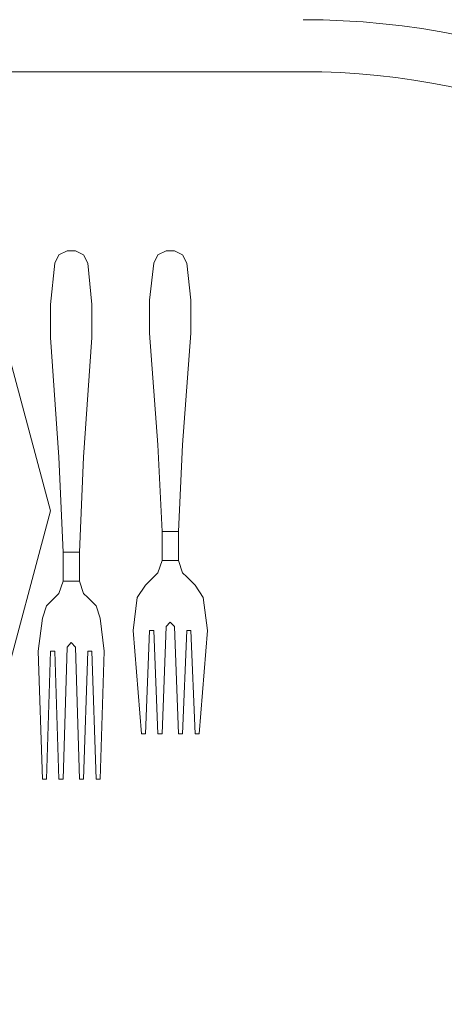
# Model space of a CAD drawing. Units: inches. Extents: x 375 to 1122, y 27 to 1069.
# Tile 146 of 155: x 731.16 to 737.5, y 901.85 to 916.52. Entities that reach past the tile are written whole.
import ezdxf

# ---------------------------------------------------------------- set-up
doc = ezdxf.new("R2010")
doc.units = ezdxf.units.IN
doc.layers.add('A-ANNO-DIMS', color=2, linetype='Continuous', lineweight=18)
doc.layers.add('Furniture', color=30, linetype='Continuous', lineweight=18)
doc.styles.get("Standard").update_dxf_attribs({"font": 'arial.ttf'})
doc.dimstyles.new('ISO-25', dxfattribs={"dimtxt": 12, "dimasz": 2.5, "dimexe": 1.5, "dimexo": 1.5, "dimtad": 1, "dimdec": 1, "dimlunit": 3, "dimtxsty": 'Standard', "dimblk": 'ARCHTICK', "dimcen": 2.5, "dimadec": 0, "dimazin": 0, "dimtfac": 1, "dimtdec": 1, "dimtmove": 0, "dimatfit": 3, "dimfxl": 1.5, "dimfxlon": 1, "dimarcsym": 0})

# ---------------------------------------------------------------- blocks, each defined once
blk = doc.blocks.new('A$C403C54AD')
for p, q in [((0.56427, 0.79569, -0.0006), (0.56427, 1.26108, -0.0006)), ((0.76029, 1.22386, -0.03201), (0.75567, 1.22078, -0.03155)), ((0.76029, 1.22386, -0.03509), (0.75567, 1.22078, -0.03463)), ((0.76798, 1.18538, -0.03201), (0.76336, 1.18384, -0.03155)), ((0.76798, 1.18538, -0.03509), (0.76336, 1.18384, -0.03463))]:
    blk.add_line(p, q)
for radius in [0.29087, 0.27148]:
    blk.add_arc((0.83575, 1.26108, -0.0006), radius, 90, 180)
for points, invisible_edges in [([(0.75567, 1.20231, -0.03155), (0.75567, 1.22078, -0.03155), (0.76029, 1.22386, -0.03201), (0.76029, 1.19923, -0.03201)], 5), ([(0.75567, 1.20231, -0.03463), (0.75567, 1.22078, -0.03463), (0.76029, 1.22386, -0.03509), (0.76029, 1.19923, -0.03509)], 5), ([(0.75567, 1.22078, -0.03155), (0.75567, 1.22078, -0.03463), (0.76029, 1.22386, -0.03509), (0.76029, 1.22386, -0.03201)], 4), ([(0.76029, 1.22386, -0.03201), (0.7726, 1.2177, -0.03141), (0.7726, 1.21924, -0.03141), (0.7726, 1.2254, -0.03141)], 5), ([(0.76029, 1.22386, -0.03509), (0.7726, 1.2177, -0.03449), (0.7726, 1.21924, -0.03449), (0.7726, 1.2254, -0.03449)], 5), ([(0.76029, 1.22386, -0.03509), (0.76029, 1.22386, -0.03201), (0.7726, 1.2254, -0.03141), (0.7726, 1.2254, -0.03449)], 1), ([(0.76029, 1.22386, -0.03201), (0.7694, 1.21155, -0.0318), (0.77106, 1.21308, -0.03166), (0.7726, 1.2177, -0.03141)], 13), ([(0.76029, 1.19923, -0.03201), (0.7694, 1.21155, -0.0318), (0.76029, 1.22386, -0.03201), (0.76029, 1.19923, -0.03201)], 7), ([(0.76029, 1.22386, -0.03509), (0.7694, 1.21155, -0.03488), (0.77106, 1.21308, -0.03473), (0.7726, 1.2177, -0.03449)], 13), ([(0.76029, 1.19923, -0.03509), (0.7694, 1.21155, -0.03488), (0.76029, 1.22386, -0.03509), (0.76029, 1.19923, -0.03509)], 7), ([(0.7726, 1.21924, -0.03141), (0.7726, 1.2254, -0.03141), (0.81108, 1.22232, -0.02431), (0.81108, 1.22078, -0.02431)], 1), ([(0.7726, 1.21924, -0.03449), (0.7726, 1.2254, -0.03449), (0.81108, 1.22232, -0.02739), (0.81108, 1.22078, -0.02739)], 1), ([(0.63561, 1.2177, -0.03041), (0.63561, 1.20539, -0.03041), (0.64946, 1.20385, -0.03045), (0.64946, 1.21924, -0.03045)], 5), ([(0.63561, 1.2177, -0.03505), (0.63561, 1.20539, -0.03505), (0.64946, 1.20385, -0.03508), (0.64946, 1.21924, -0.03508)], 5), ([(0.64946, 1.20385, -0.03045), (0.64946, 1.21924, -0.03045), (0.66178, 1.21924, -0.03012), (0.66178, 1.20385, -0.03012)], 5), ([(0.64946, 1.20385, -0.03508), (0.64946, 1.21924, -0.03508), (0.66178, 1.21924, -0.03476), (0.66178, 1.20385, -0.03476)], 5), ([(0.66178, 1.21924, -0.03012), (0.66178, 1.20385, -0.03012), (0.70334, 1.20693, -0.02774), (0.70334, 1.21616, -0.02774)], 5), ([(0.66178, 1.21924, -0.03476), (0.66178, 1.20385, -0.03476), (0.70334, 1.20693, -0.03082), (0.70334, 1.21616, -0.03082)], 5), ([(0.70334, 1.21616, -0.03082), (0.70334, 1.21616, -0.02774), (0.66178, 1.21924, -0.03012), (0.66178, 1.21924, -0.03476)], 1), ([(0.75259, 1.2177, -0.03339), (0.75259, 1.20539, -0.03339), (0.75567, 1.20231, -0.03463), (0.75567, 1.22078, -0.03463)], 5), ([(0.75259, 1.2177, -0.03031), (0.75259, 1.20539, -0.03031), (0.75567, 1.20231, -0.03155), (0.75567, 1.22078, -0.03155)], 5), ([(0.63099, 1.21308, -0.03034), (0.63099, 1.21001, -0.03034), (0.63253, 1.20693, -0.03017), (0.63253, 1.21616, -0.03017)], 4), ([(0.63099, 1.21308, -0.03447), (0.63099, 1.21001, -0.03447), (0.63253, 1.20693, -0.03481), (0.63253, 1.21616, -0.03481)], 4), ([(0.63253, 1.20693, -0.03017), (0.63253, 1.21616, -0.03017), (0.63561, 1.2177, -0.03041), (0.63561, 1.20539, -0.03041)], 5), ([(0.63253, 1.20693, -0.03481), (0.63253, 1.21616, -0.03481), (0.63561, 1.2177, -0.03505), (0.63561, 1.20539, -0.03505)], 5), ([(0.70334, 1.20693, -0.02774), (0.70334, 1.21616, -0.02774), (0.73566, 1.21462, -0.02483), (0.73566, 1.20847, -0.02483)], 1), ([(0.73566, 1.21462, -0.02483), (0.73566, 1.21462, -0.02742), (0.70334, 1.21616, -0.03082), (0.70334, 1.21616, -0.02774)], 5), ([(0.70334, 1.20693, -0.03082), (0.70334, 1.21616, -0.03082), (0.73566, 1.21462, -0.02742), (0.73566, 1.20847, -0.02742)], 1), ([(0.74643, 1.20847, -0.02691), (0.74643, 1.21462, -0.02691), (0.75105, 1.21616, -0.02926), (0.75105, 1.20693, -0.02926)], 4), ([(0.74643, 1.20847, -0.0295), (0.74643, 1.21462, -0.0295), (0.75105, 1.21616, -0.03205), (0.75105, 1.20693, -0.03205)], 4), ([(0.74643, 1.21462, -0.0295), (0.74643, 1.21462, -0.02691), (0.75105, 1.21616, -0.02926), (0.75105, 1.21616, -0.03205)], 5), ([(0.75105, 1.21616, -0.02926), (0.75105, 1.20693, -0.02926), (0.75259, 1.20539, -0.03031), (0.75259, 1.2177, -0.03031)], 5), ([(0.75105, 1.21616, -0.03205), (0.75105, 1.20693, -0.03205), (0.75259, 1.20539, -0.03339), (0.75259, 1.2177, -0.03339)], 5), ([(0.75105, 1.21616, -0.02926), (0.75105, 1.21616, -0.03205), (0.75259, 1.2177, -0.03339), (0.75259, 1.2177, -0.03031)], 1), ([(0.77106, 1.21308, -0.03166), (0.7726, 1.2177, -0.03141), (0.81108, 1.21616, -0.02431), (0.81108, 1.21462, -0.02431)], 1), ([(0.77106, 1.21308, -0.03473), (0.7726, 1.2177, -0.03449), (0.81108, 1.21616, -0.02739), (0.81108, 1.21462, -0.02739)], 1), ([(0.74643, 1.21462, -0.0295), (0.74643, 1.21462, -0.02691), (0.73566, 1.21462, -0.02483), (0.73566, 1.21462, -0.02742)], 5), ([(0.76029, 1.19923, -0.03201), (0.7694, 1.21155, -0.0318), (0.77106, 1.21001, -0.03166), (0.7726, 1.20539, -0.03141)], 13), ([(0.76029, 1.19923, -0.03509), (0.7694, 1.21155, -0.03488), (0.77106, 1.21001, -0.03473), (0.7726, 1.20539, -0.03449)], 13), ([(0.70334, 1.20693, -0.02774), (0.70334, 1.20693, -0.03082), (0.73566, 1.20847, -0.02742), (0.73566, 1.20847, -0.02483)], 5), ([(0.73566, 1.20847, -0.02742), (0.73566, 1.20847, -0.02483), (0.74643, 1.20847, -0.02691), (0.74643, 1.20847, -0.0295)], 5), ([(0.74643, 1.20847, -0.02691), (0.74643, 1.20847, -0.0295), (0.75105, 1.20693, -0.03205), (0.75105, 1.20693, -0.02926)], 5), ([(0.7726, 1.20539, -0.03141), (0.77106, 1.21001, -0.03166), (0.81108, 1.20847, -0.02431), (0.81108, 1.20693, -0.02431)], 1), ([(0.7726, 1.20539, -0.03449), (0.77106, 1.21001, -0.03473), (0.81108, 1.20847, -0.02739), (0.81108, 1.20693, -0.02739)], 1), ([(0.66178, 1.20385, -0.03476), (0.66178, 1.20385, -0.03012), (0.70334, 1.20693, -0.02774), (0.70334, 1.20693, -0.03082)], 4), ([(0.75105, 1.20693, -0.03205), (0.75105, 1.20693, -0.02926), (0.75259, 1.20539, -0.03031), (0.75259, 1.20539, -0.03339)], 1), ([(0.76029, 1.19923, -0.03201), (0.7726, 1.20539, -0.03141), (0.7726, 1.20385, -0.03141), (0.7726, 1.19769, -0.03141)], 5), ([(0.76029, 1.19923, -0.03509), (0.7726, 1.20539, -0.03449), (0.7726, 1.20385, -0.03449), (0.7726, 1.19769, -0.03449)], 5), ([(0.7726, 1.20385, -0.03141), (0.7726, 1.19769, -0.03141), (0.81108, 1.20077, -0.02431), (0.81108, 1.20231, -0.02431)], 1), ([(0.7726, 1.20385, -0.03449), (0.7726, 1.19769, -0.03449), (0.81108, 1.20077, -0.02739), (0.81108, 1.20231, -0.02739)], 1), ([(0.75567, 1.20231, -0.03463), (0.75567, 1.20231, -0.03155), (0.76029, 1.19923, -0.03201), (0.76029, 1.19923, -0.03509)], 4), ([(0.76029, 1.19923, -0.03201), (0.76029, 1.19923, -0.03509), (0.7726, 1.19769, -0.03449), (0.7726, 1.19769, -0.03141)], 1), ([(0.76798, 1.18538, -0.03201), (0.7803, 1.18076, -0.03141), (0.7803, 1.1823, -0.03141), (0.7803, 1.18692, -0.03141)], 5), ([(0.76798, 1.18538, -0.03509), (0.7803, 1.18076, -0.03449), (0.7803, 1.1823, -0.03449), (0.7803, 1.18692, -0.03449)], 5), ([(0.76798, 1.18538, -0.03509), (0.76798, 1.18538, -0.03201), (0.7803, 1.18692, -0.03141), (0.7803, 1.18692, -0.03449)], 1), ([(0.7803, 1.1823, -0.03141), (0.7803, 1.18692, -0.03141), (0.82801, 1.18538, -0.02431), (0.82801, 1.18384, -0.02431)], 1), ([(0.7803, 1.1823, -0.03449), (0.7803, 1.18692, -0.03449), (0.82801, 1.18538, -0.02739), (0.82801, 1.18384, -0.02739)], 1), ([(0.63561, 1.18076, -0.03041), (0.63561, 1.16845, -0.03041), (0.651, 1.16691, -0.03045), (0.651, 1.1823, -0.03045)], 5), ([(0.63561, 1.18076, -0.03505), (0.63561, 1.16845, -0.03505), (0.651, 1.16691, -0.03508), (0.651, 1.1823, -0.03508)], 5), ([(0.651, 1.16691, -0.03045), (0.651, 1.1823, -0.03045), (0.66332, 1.1823, -0.03012), (0.66332, 1.16691, -0.03012)], 5), ([(0.651, 1.16691, -0.03508), (0.651, 1.1823, -0.03508), (0.66332, 1.1823, -0.03476), (0.66332, 1.16691, -0.03476)], 5), ([(0.66332, 1.1823, -0.03012), (0.66332, 1.16691, -0.03012), (0.70795, 1.16999, -0.02774), (0.70795, 1.17922, -0.02774)], 5), ([(0.66332, 1.1823, -0.03476), (0.66332, 1.16691, -0.03476), (0.70795, 1.16999, -0.03082), (0.70795, 1.17922, -0.03082)], 5), ([(0.70795, 1.17922, -0.03082), (0.70795, 1.17922, -0.02774), (0.66332, 1.1823, -0.03012), (0.66332, 1.1823, -0.03476)], 1), ([(0.76029, 1.18076, -0.03339), (0.76029, 1.16845, -0.03339), (0.76336, 1.16537, -0.03463), (0.76336, 1.18384, -0.03463)], 5), ([(0.76029, 1.18076, -0.03031), (0.76029, 1.16845, -0.03031), (0.76336, 1.16537, -0.03155), (0.76336, 1.18384, -0.03155)], 5), ([(0.76336, 1.16537, -0.03155), (0.76336, 1.18384, -0.03155), (0.76798, 1.18538, -0.03201), (0.76798, 1.16383, -0.03201)], 5), ([(0.76336, 1.16537, -0.03463), (0.76336, 1.18384, -0.03463), (0.76798, 1.18538, -0.03509), (0.76798, 1.16383, -0.03509)], 5), ([(0.76336, 1.18384, -0.03155), (0.76336, 1.18384, -0.03463), (0.76798, 1.18538, -0.03509), (0.76798, 1.18538, -0.03201)], 4), ([(0.76798, 1.18538, -0.03201), (0.77709, 1.17461, -0.0318), (0.77876, 1.17614, -0.03166), (0.7803, 1.18076, -0.03141)], 13), ([(0.76798, 1.16383, -0.03201), (0.77709, 1.17461, -0.0318), (0.76798, 1.18538, -0.03201), (0.76798, 1.16383, -0.03201)], 7), ([(0.76798, 1.16383, -0.03509), (0.77709, 1.17461, -0.03488), (0.76798, 1.18538, -0.03509), (0.76798, 1.16383, -0.03509)], 7), ([(0.76798, 1.18538, -0.03509), (0.77709, 1.17461, -0.03488), (0.77876, 1.17614, -0.03473), (0.7803, 1.18076, -0.03449)], 13), ([(0.63099, 1.17614, -0.03034), (0.63099, 1.17307, -0.03034), (0.63253, 1.16999, -0.03017), (0.63253, 1.17922, -0.03017)], 4), ([(0.63099, 1.17614, -0.03447), (0.63099, 1.17307, -0.03447), (0.63253, 1.16999, -0.03481), (0.63253, 1.17922, -0.03481)], 4), ([(0.63253, 1.16999, -0.03017), (0.63253, 1.17922, -0.03017), (0.63561, 1.18076, -0.03041), (0.63561, 1.16845, -0.03041)], 5), ([(0.63253, 1.16999, -0.03481), (0.63253, 1.17922, -0.03481), (0.63561, 1.18076, -0.03505), (0.63561, 1.16845, -0.03505)], 5), ([(0.70795, 1.16999, -0.02774), (0.70795, 1.17922, -0.02774), (0.74335, 1.17768, -0.02483), (0.74335, 1.17153, -0.02483)], 1), ([(0.74335, 1.17768, -0.02483), (0.74335, 1.17768, -0.02742), (0.70795, 1.17922, -0.03082), (0.70795, 1.17922, -0.02774)], 5), ([(0.70795, 1.16999, -0.03082), (0.70795, 1.17922, -0.03082), (0.74335, 1.17768, -0.02742), (0.74335, 1.17153, -0.02742)], 1), ([(0.75413, 1.17153, -0.02691), (0.75413, 1.17768, -0.02691), (0.75875, 1.17922, -0.02926), (0.75875, 1.16999, -0.02926)], 4), ([(0.75413, 1.17768, -0.0295), (0.75413, 1.17768, -0.02691), (0.75875, 1.17922, -0.02926), (0.75875, 1.17922, -0.03205)], 5), ([(0.75413, 1.17153, -0.0295), (0.75413, 1.17768, -0.0295), (0.75875, 1.17922, -0.03205), (0.75875, 1.16999, -0.03205)], 4), ([(0.75875, 1.17922, -0.02926), (0.75875, 1.16999, -0.02926), (0.76029, 1.16845, -0.03031), (0.76029, 1.18076, -0.03031)], 5), ([(0.75875, 1.17922, -0.03205), (0.75875, 1.16999, -0.03205), (0.76029, 1.16845, -0.03339), (0.76029, 1.18076, -0.03339)], 5), ([(0.75875, 1.17922, -0.02926), (0.75875, 1.17922, -0.03205), (0.76029, 1.18076, -0.03339), (0.76029, 1.18076, -0.03031)], 1), ([(0.77876, 1.17614, -0.03166), (0.7803, 1.18076, -0.03141), (0.82801, 1.17922, -0.02431), (0.82801, 1.17768, -0.02431)], 1), ([(0.77876, 1.17614, -0.03473), (0.7803, 1.18076, -0.03449), (0.82801, 1.17922, -0.02739), (0.82801, 1.17768, -0.02739)], 1), ([(0.75413, 1.17768, -0.0295), (0.75413, 1.17768, -0.02691), (0.74335, 1.17768, -0.02483), (0.74335, 1.17768, -0.02742)], 5), ([(0.76798, 1.16383, -0.03201), (0.77709, 1.17461, -0.0318), (0.77876, 1.17307, -0.03166), (0.7803, 1.16845, -0.03141)], 13), ([(0.76798, 1.16383, -0.03509), (0.77709, 1.17461, -0.03488), (0.77876, 1.17307, -0.03473), (0.7803, 1.16845, -0.03449)], 13), ([(0.70795, 1.16999, -0.02774), (0.70795, 1.16999, -0.03082), (0.74335, 1.17153, -0.02742), (0.74335, 1.17153, -0.02483)], 5), ([(0.74335, 1.17153, -0.02742), (0.74335, 1.17153, -0.02483), (0.75413, 1.17153, -0.02691), (0.75413, 1.17153, -0.0295)], 5), ([(0.75413, 1.17153, -0.02691), (0.75413, 1.17153, -0.0295), (0.75875, 1.16999, -0.03205), (0.75875, 1.16999, -0.02926)], 5), ([(0.7803, 1.16845, -0.03141), (0.77876, 1.17307, -0.03166), (0.82801, 1.17153, -0.02431), (0.82801, 1.16999, -0.02431)], 1), ([(0.7803, 1.16845, -0.03449), (0.77876, 1.17307, -0.03473), (0.82801, 1.17153, -0.02739), (0.82801, 1.16999, -0.02739)], 1), ([(0.66332, 1.16691, -0.03476), (0.66332, 1.16691, -0.03012), (0.70795, 1.16999, -0.02774), (0.70795, 1.16999, -0.03082)], 4), ([(0.75875, 1.16999, -0.03205), (0.75875, 1.16999, -0.02926), (0.76029, 1.16845, -0.03031), (0.76029, 1.16845, -0.03339)], 1), ([(0.76798, 1.16383, -0.03201), (0.7803, 1.16845, -0.03141), (0.7803, 1.16691, -0.03141), (0.7803, 1.16229, -0.03141)], 5), ([(0.76798, 1.16383, -0.03509), (0.7803, 1.16845, -0.03449), (0.7803, 1.16691, -0.03449), (0.7803, 1.16229, -0.03449)], 5), ([(0.76336, 1.16537, -0.03463), (0.76336, 1.16537, -0.03155), (0.76798, 1.16383, -0.03201), (0.76798, 1.16383, -0.03509)], 4), ([(0.76798, 1.16383, -0.03201), (0.76798, 1.16383, -0.03509), (0.7803, 1.16229, -0.03449), (0.7803, 1.16229, -0.03141)], 1), ([(0.7803, 1.16691, -0.03141), (0.7803, 1.16229, -0.03141), (0.82801, 1.16383, -0.02431), (0.82801, 1.16537, -0.02431)], 1), ([(0.7803, 1.16691, -0.03449), (0.7803, 1.16229, -0.03449), (0.82801, 1.16383, -0.02739), (0.82801, 1.16537, -0.02739)], 1)]:
    blk.add_3dface(points, dxfattribs=dict(invisible_edges=invisible_edges))
for points in [[(0.81108, 1.22232, -0.02431), (0.81108, 1.22232, -0.02739), (0.7726, 1.2254, -0.03449), (0.7726, 1.2254, -0.03141)], [(0.81108, 1.22078, -0.02739), (0.81108, 1.22078, -0.02431), (0.81108, 1.22232, -0.02431), (0.81108, 1.22232, -0.02739)], [(0.64946, 1.21924, -0.03508), (0.64946, 1.21924, -0.03045), (0.63561, 1.2177, -0.03041), (0.63561, 1.2177, -0.03505)], [(0.66178, 1.21924, -0.03012), (0.66178, 1.21924, -0.03476), (0.64946, 1.21924, -0.03508), (0.64946, 1.21924, -0.03045)], [(0.75259, 1.2177, -0.03339), (0.75259, 1.2177, -0.03031), (0.75567, 1.22078, -0.03155), (0.75567, 1.22078, -0.03463)], [(0.7726, 1.21924, -0.03141), (0.7726, 1.21924, -0.03449), (0.81108, 1.22078, -0.02739), (0.81108, 1.22078, -0.02431)], [(0.7726, 1.21924, -0.03141), (0.7726, 1.21924, -0.03449), (0.7726, 1.2177, -0.03449), (0.7726, 1.2177, -0.03141)], [(0.63253, 1.21616, -0.03481), (0.63253, 1.21616, -0.03017), (0.63099, 1.21308, -0.03034), (0.63099, 1.21308, -0.03447)], [(0.63561, 1.2177, -0.03041), (0.63561, 1.2177, -0.03505), (0.63253, 1.21616, -0.03481), (0.63253, 1.21616, -0.03017)], [(0.81108, 1.21616, -0.02431), (0.81108, 1.21616, -0.02739), (0.7726, 1.2177, -0.03449), (0.7726, 1.2177, -0.03141)], [(0.81108, 1.21462, -0.02739), (0.81108, 1.21462, -0.02431), (0.81108, 1.21616, -0.02431), (0.81108, 1.21616, -0.02739)], [(0.63099, 1.21308, -0.03034), (0.63099, 1.21308, -0.03447), (0.63099, 1.21001, -0.03447), (0.63099, 1.21001, -0.03034)], [(0.73566, 1.21462, -0.02483), (0.73566, 1.20847, -0.02483), (0.74643, 1.20847, -0.02691), (0.74643, 1.21462, -0.02691)], [(0.73566, 1.21462, -0.02742), (0.73566, 1.20847, -0.02742), (0.74643, 1.20847, -0.0295), (0.74643, 1.21462, -0.0295)], [(0.77106, 1.21308, -0.03166), (0.77106, 1.21308, -0.03473), (0.7694, 1.21155, -0.03488), (0.7694, 1.21155, -0.0318)], [(0.7694, 1.21155, -0.03488), (0.7694, 1.21155, -0.0318), (0.77106, 1.21001, -0.03166), (0.77106, 1.21001, -0.03473)], [(0.77106, 1.21308, -0.03473), (0.77106, 1.21308, -0.03166), (0.81108, 1.21462, -0.02431), (0.81108, 1.21462, -0.02739)], [(0.63099, 1.21001, -0.03447), (0.63099, 1.21001, -0.03034), (0.63253, 1.20693, -0.03017), (0.63253, 1.20693, -0.03481)], [(0.81108, 1.20847, -0.02739), (0.81108, 1.20847, -0.02431), (0.77106, 1.21001, -0.03166), (0.77106, 1.21001, -0.03473)], [(0.81108, 1.20693, -0.02739), (0.81108, 1.20693, -0.02431), (0.81108, 1.20847, -0.02431), (0.81108, 1.20847, -0.02739)], [(0.63253, 1.20693, -0.03017), (0.63253, 1.20693, -0.03481), (0.63561, 1.20539, -0.03505), (0.63561, 1.20539, -0.03041)], [(0.63561, 1.20539, -0.03505), (0.63561, 1.20539, -0.03041), (0.64946, 1.20385, -0.03045), (0.64946, 1.20385, -0.03508)], [(0.64946, 1.20385, -0.03045), (0.64946, 1.20385, -0.03508), (0.66178, 1.20385, -0.03476), (0.66178, 1.20385, -0.03012)], [(0.75259, 1.20539, -0.03031), (0.75259, 1.20539, -0.03339), (0.75567, 1.20231, -0.03463), (0.75567, 1.20231, -0.03155)], [(0.7726, 1.20539, -0.03449), (0.7726, 1.20539, -0.03141), (0.81108, 1.20693, -0.02431), (0.81108, 1.20693, -0.02739)], [(0.7726, 1.20539, -0.03449), (0.7726, 1.20539, -0.03141), (0.7726, 1.20385, -0.03141), (0.7726, 1.20385, -0.03449)], [(0.81108, 1.20231, -0.02431), (0.81108, 1.20231, -0.02739), (0.7726, 1.20385, -0.03449), (0.7726, 1.20385, -0.03141)], [(0.7726, 1.19769, -0.03449), (0.7726, 1.19769, -0.03141), (0.81108, 1.20077, -0.02431), (0.81108, 1.20077, -0.02739)], [(0.81108, 1.20077, -0.02739), (0.81108, 1.20077, -0.02431), (0.81108, 1.20231, -0.02431), (0.81108, 1.20231, -0.02739)], [(0.82801, 1.18538, -0.02431), (0.82801, 1.18538, -0.02739), (0.7803, 1.18692, -0.03449), (0.7803, 1.18692, -0.03141)], [(0.651, 1.1823, -0.03508), (0.651, 1.1823, -0.03045), (0.63561, 1.18076, -0.03041), (0.63561, 1.18076, -0.03505)], [(0.66332, 1.1823, -0.03012), (0.66332, 1.1823, -0.03476), (0.651, 1.1823, -0.03508), (0.651, 1.1823, -0.03045)], [(0.76029, 1.18076, -0.03339), (0.76029, 1.18076, -0.03031), (0.76336, 1.18384, -0.03155), (0.76336, 1.18384, -0.03463)], [(0.7803, 1.1823, -0.03141), (0.7803, 1.1823, -0.03449), (0.82801, 1.18384, -0.02739), (0.82801, 1.18384, -0.02431)], [(0.7803, 1.1823, -0.03141), (0.7803, 1.1823, -0.03449), (0.7803, 1.18076, -0.03449), (0.7803, 1.18076, -0.03141)], [(0.82801, 1.18384, -0.02739), (0.82801, 1.18384, -0.02431), (0.82801, 1.18538, -0.02431), (0.82801, 1.18538, -0.02739)], [(0.63253, 1.17922, -0.03481), (0.63253, 1.17922, -0.03017), (0.63099, 1.17614, -0.03034), (0.63099, 1.17614, -0.03447)], [(0.63561, 1.18076, -0.03041), (0.63561, 1.18076, -0.03505), (0.63253, 1.17922, -0.03481), (0.63253, 1.17922, -0.03017)], [(0.82801, 1.17922, -0.02431), (0.82801, 1.17922, -0.02739), (0.7803, 1.18076, -0.03449), (0.7803, 1.18076, -0.03141)], [(0.82801, 1.17768, -0.02739), (0.82801, 1.17768, -0.02431), (0.82801, 1.17922, -0.02431), (0.82801, 1.17922, -0.02739)], [(0.63099, 1.17614, -0.03034), (0.63099, 1.17614, -0.03447), (0.63099, 1.17307, -0.03447), (0.63099, 1.17307, -0.03034)], [(0.74335, 1.17768, -0.02483), (0.74335, 1.17153, -0.02483), (0.75413, 1.17153, -0.02691), (0.75413, 1.17768, -0.02691)], [(0.74335, 1.17768, -0.02742), (0.74335, 1.17153, -0.02742), (0.75413, 1.17153, -0.0295), (0.75413, 1.17768, -0.0295)], [(0.77876, 1.17614, -0.03166), (0.77876, 1.17614, -0.03473), (0.77709, 1.17461, -0.03488), (0.77709, 1.17461, -0.0318)], [(0.77709, 1.17461, -0.03488), (0.77709, 1.17461, -0.0318), (0.77876, 1.17307, -0.03166), (0.77876, 1.17307, -0.03473)], [(0.77876, 1.17614, -0.03473), (0.77876, 1.17614, -0.03166), (0.82801, 1.17768, -0.02431), (0.82801, 1.17768, -0.02739)], [(0.63099, 1.17307, -0.03447), (0.63099, 1.17307, -0.03034), (0.63253, 1.16999, -0.03017), (0.63253, 1.16999, -0.03481)], [(0.82801, 1.17153, -0.02739), (0.82801, 1.17153, -0.02431), (0.77876, 1.17307, -0.03166), (0.77876, 1.17307, -0.03473)], [(0.82801, 1.16999, -0.02739), (0.82801, 1.16999, -0.02431), (0.82801, 1.17153, -0.02431), (0.82801, 1.17153, -0.02739)], [(0.63253, 1.16999, -0.03017), (0.63253, 1.16999, -0.03481), (0.63561, 1.16845, -0.03505), (0.63561, 1.16845, -0.03041)], [(0.63561, 1.16845, -0.03505), (0.63561, 1.16845, -0.03041), (0.651, 1.16691, -0.03045), (0.651, 1.16691, -0.03508)], [(0.76029, 1.16845, -0.03031), (0.76029, 1.16845, -0.03339), (0.76336, 1.16537, -0.03463), (0.76336, 1.16537, -0.03155)], [(0.7803, 1.16845, -0.03449), (0.7803, 1.16845, -0.03141), (0.82801, 1.16999, -0.02431), (0.82801, 1.16999, -0.02739)], [(0.7803, 1.16845, -0.03449), (0.7803, 1.16845, -0.03141), (0.7803, 1.16691, -0.03141), (0.7803, 1.16691, -0.03449)], [(0.651, 1.16691, -0.03045), (0.651, 1.16691, -0.03508), (0.66332, 1.16691, -0.03476), (0.66332, 1.16691, -0.03012)], [(0.82801, 1.16537, -0.02431), (0.82801, 1.16537, -0.02739), (0.7803, 1.16691, -0.03449), (0.7803, 1.16691, -0.03141)], [(0.7803, 1.16229, -0.03449), (0.7803, 1.16229, -0.03141), (0.82801, 1.16383, -0.02431), (0.82801, 1.16383, -0.02739)], [(0.82801, 1.16383, -0.02739), (0.82801, 1.16383, -0.02431), (0.82801, 1.16537, -0.02431), (0.82801, 1.16537, -0.02739)]]:
    blk.add_3dface(points)
at = {"linetype": 'ByBlock', "invisible_edges": 5}
for points in [[(0.72796, 1.16691, -0.0197), (0.72796, 1.14844, -0.0197), (0.66793, 1.13235, -0.0197), (0.6587, 1.14835, -0.0197)], [(0.72796, 1.13305, -0.03355), (0.72796, 1.16691, -0.02431), (0.6587, 1.14835, -0.02431), (0.67563, 1.11902, -0.03355)], [(0.79723, 1.14835, -0.0197), (0.78799, 1.13235, -0.0197), (0.72796, 1.14844, -0.0197), (0.72796, 1.16691, -0.0197)], [(0.7803, 1.11902, -0.03355), (0.79723, 1.14835, -0.02431), (0.72796, 1.16691, -0.02431), (0.72796, 1.13305, -0.03355)]]:
    blk.add_3dface(points, dxfattribs=at)
at = {"linetype": 'ByBlock'}
for points in [[(0.72796, 1.16691, -0.02431), (0.72796, 1.16691, -0.0197), (0.6587, 1.14835, -0.0197), (0.6587, 1.14835, -0.02431)], [(0.79723, 1.14835, -0.02431), (0.79723, 1.14835, -0.0197), (0.72796, 1.16691, -0.0197), (0.72796, 1.16691, -0.02431)]]:
    blk.add_3dface(points, dxfattribs=at)
blk = doc.blocks.new('_ArchTick')
at = {"color": 0, "linetype": 'ByBlock', "const_width": 0.15}
blk.add_lwpolyline([(-0.5, -0.5), (0.5, 0.5)], dxfattribs=at)
blk = doc.blocks.new('*D73')
at = {"layer": 'A-ANNO-DIMS', "color": 0, "lineweight": -2, "transparency": 16777216}
for p, q in [((686.757, 932.428), (686.757, 929.428)), ((770.757, 932.428), (770.757, 929.428)), ((686.757, 930.928), (770.757, 930.928)), ((770.757, 930.928), (987.61, 930.928))]:
    blk.add_line(p, q, dxfattribs=at)
at = {"layer": 'Defpoints', "color": 0, "transparency": 16777216}
for p in [(686.757, 943.528), (770.757, 943.528), (770.757, 930.928)]:
    blk.add_point(p, dxfattribs=at)
at = {"layer": 'A-ANNO-DIMS', "color": 0, "lineweight": -2, "transparency": 16777216, "xscale": 2.5, "yscale": 2.5, "zscale": 2.5, "rotation": 180}
blk.add_blockref('_ArchTick', (686.757, 930.928), dxfattribs=at)
at = {"layer": 'A-ANNO-DIMS', "color": 0, "lineweight": -2, "transparency": 16777216, "xscale": 2.5, "yscale": 2.5, "zscale": 2.5}
blk.add_blockref('_ArchTick', (770.757, 930.928), dxfattribs=at)
at = {"layer": 'A-ANNO-DIMS', "color": 0, "transparency": 16777216, "insert": (880.433, 937.757), "char_height": 12, "attachment_point": 5}
blk.add_mtext('2-PANEL SLIDER 7\'-0" TYP.', dxfattribs=at)
blk = doc.blocks.new('*D88')
at = {"layer": 'A-ANNO-DIMS', "color": 0, "lineweight": -2, "transparency": 16777216}
for p, q in [((731.007, 1052.528), (731.007, 1055.528)), ((854.007, 1052.528), (854.007, 1055.528)), ((731.007, 1054.028), (854.007, 1054.028))]:
    blk.add_line(p, q, dxfattribs=at)
at = {"layer": 'Defpoints', "color": 0, "transparency": 16777216}
for p in [(854.007, 1054.028), (731.007, 502.528), (854.007, 502.528)]:
    blk.add_point(p, dxfattribs=at)
at = {"layer": 'A-ANNO-DIMS', "color": 0, "lineweight": -2, "transparency": 16777216, "xscale": 2.5, "yscale": 2.5, "zscale": 2.5, "rotation": 180}
blk.add_blockref('_ArchTick', (731.007, 1054.028), dxfattribs=at)
at = {"layer": 'A-ANNO-DIMS', "color": 0, "lineweight": -2, "transparency": 16777216, "xscale": 2.5, "yscale": 2.5, "zscale": 2.5}
blk.add_blockref('_ArchTick', (854.007, 1054.028), dxfattribs=at)
at = {"layer": 'A-ANNO-DIMS', "color": 0, "transparency": 16777216, "insert": (792.507, 1060.784), "char_height": 12, "attachment_point": 5}
blk.add_mtext('10\'-3"', dxfattribs=at)
blk = doc.blocks.new('*D91')
at = {"layer": 'A-ANNO-DIMS', "color": 0, "lineweight": -2, "transparency": 16777216}
for p, q in [((728.007, 1052.528), (728.007, 1055.528)), ((788.007, 1052.528), (788.007, 1055.528)), ((728.007, 1054.028), (788.007, 1054.028))]:
    blk.add_line(p, q, dxfattribs=at)
at = {"layer": 'Defpoints', "color": 0, "transparency": 16777216}
for p in [(788.007, 1054.028), (728.007, 774.028), (788.007, 774.028)]:
    blk.add_point(p, dxfattribs=at)
at = {"layer": 'A-ANNO-DIMS', "color": 0, "lineweight": -2, "transparency": 16777216, "xscale": 2.5, "yscale": 2.5, "zscale": 2.5, "rotation": 180}
blk.add_blockref('_ArchTick', (728.007, 1054.028), dxfattribs=at)
at = {"layer": 'A-ANNO-DIMS', "color": 0, "lineweight": -2, "transparency": 16777216, "xscale": 2.5, "yscale": 2.5, "zscale": 2.5}
blk.add_blockref('_ArchTick', (788.007, 1054.028), dxfattribs=at)
at = {"layer": 'A-ANNO-DIMS', "color": 0, "transparency": 16777216, "insert": (758.007, 1060.78), "char_height": 12, "attachment_point": 5}
blk.add_mtext('5\'-0"', dxfattribs=at)

msp = doc.modelspace()

# ---------------------------------------------------------------- block references
at = {"layer": 'Furniture', "xscale": 39.9918517141215, "yscale": 39.9918517141215, "zscale": 39.9918517141215, "rotation": 270}
msp.add_blockref('A$C403C54AD', (684.955, 938.316, 0.024), dxfattribs=at)

# ---------------------------------------------------------------- dimensions: what is measured, and where the dimension line sits
at = {"layer": 'A-ANNO-DIMS'}
for base, p1, p2, picture, middle in [((788.007, 1054.028), (728.007, 774.028), (788.007, 774.028), '*D91', (758.007, 1060.78)), ((854.007, 1054.028), (731.007, 502.528), (854.007, 502.528), '*D88', (792.507, 1060.784))]:
    dim = msp.add_linear_dim(base=base, p1=p1, p2=p2, dimstyle='ISO-25', override={"dimdec": 1, "dimlfac": 1, "dimrnd": 0, "dimzin": 1, "dimdsep": 46, "dimlunit": 4, "dimfrac": 2}, dxfattribs=at)
    dim.commit()
    dim.dimension.update_dxf_attribs({"geometry": picture, "text_midpoint": middle})
dim = msp.add_linear_dim(base=(770.757, 930.928), p1=(686.757, 943.528), p2=(770.757, 943.528), text='2-PANEL SLIDER <> TYP.', dimstyle='ISO-25', override={"dimdec": 1, "dimlfac": 1, "dimrnd": 0, "dimzin": 1, "dimdsep": 46, "dimlunit": 4, "dimfrac": 2}, dxfattribs=at)
dim.commit()
dim.dimension.update_dxf_attribs({"geometry": '*D73', "text_midpoint": (880.433, 937.757)})

doc.saveas('drawing.dxf')
